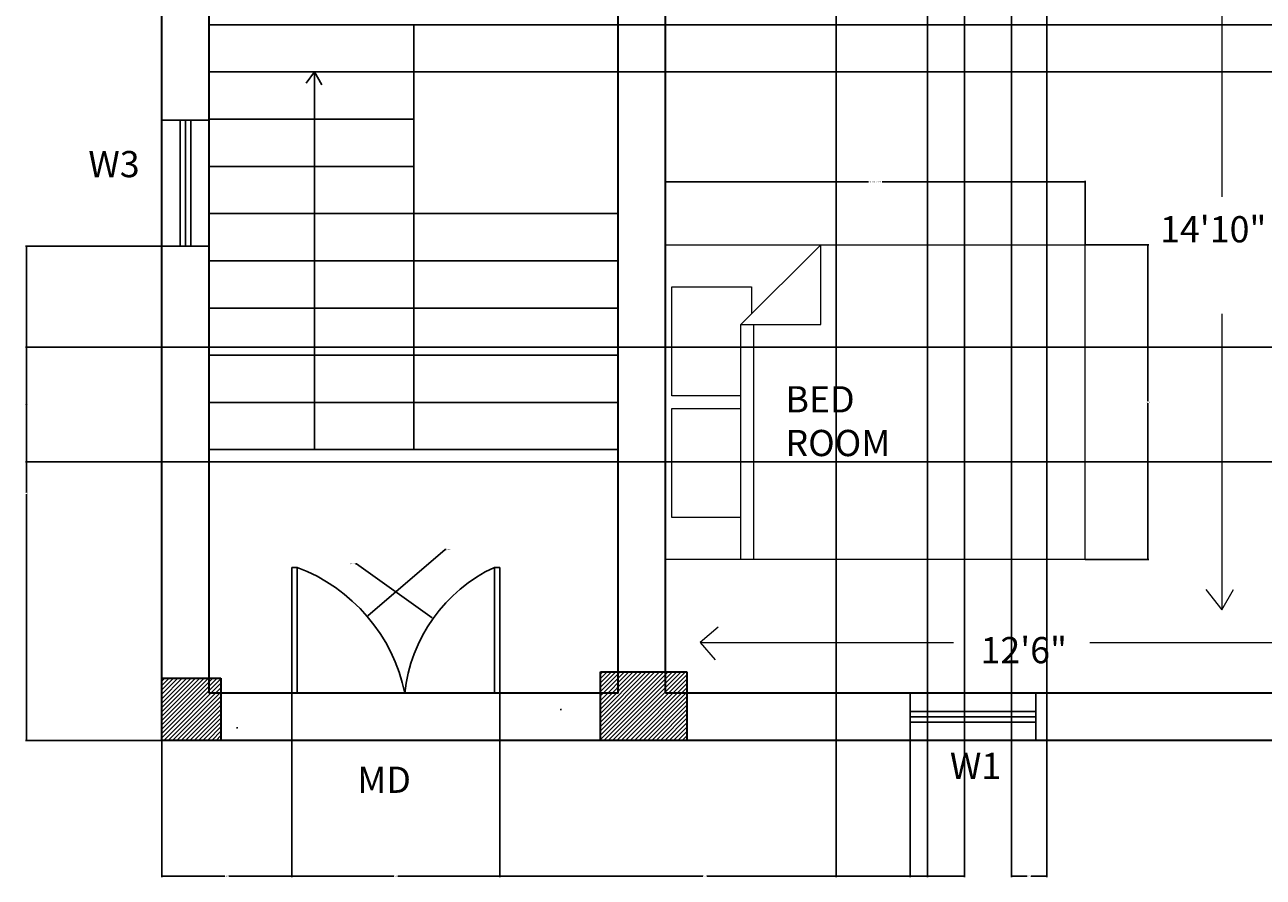
# Model space of a CAD drawing. Units: inches. Extents: x -4 to 429, y -457 to 84.
# Tile 1 of 4: x -4 to 232, y -457 to -295. Entities that reach past the tile are written whole.
import ezdxf

# ---------------------------------------------------------------- set-up
doc = ezdxf.new("R2010")
doc.units = ezdxf.units.IN
doc.header["$MEASUREMENT"] = 0
for name, color, linetype, lineweight in [('A-ANNO-DIMS', 2, 'Continuous', 18), ('A-ANNO-TEXT', 3, 'Continuous', 18), ('A-AREA-IDEN', 7, 'Continuous', 25), ('A-COLS', 7, 'Continuous', 35), ('A-COLS-PATT', 252, 'Continuous', 13), ('A-DOOR', 3, 'Continuous', 25), ('A-FLOR-STRS', 7, 'Continuous', 25), ('A-FURN', 8, 'Continuous', 18), ('A-GLAZ', 4, 'Continuous', 25), ('A-WALL', 7, 'Continuous', 35)]:
    doc.layers.add(name, color=color, linetype=linetype, lineweight=lineweight)
doc.styles.get("Standard").update_dxf_attribs({"font": 'arial.ttf'})
doc.dimstyles.get("Standard").update_dxf_attribs({"dimtxt": 0.18, "dimasz": 0.18, "dimexe": 0.18, "dimexo": 0.0625, "dimgap": 0.09, "dimtad": 0, "dimtih": 1, "dimtoh": 1, "dimdec": 4, "dimzin": 0, "dimdsep": 46, "dimtxsty": 'Standard', "dimcen": 0.09, "dimadec": 0, "dimazin": 0, "dimtfac": 1, "dimtdec": 4, "dimtofl": 0, "dimtmove": 0, "dimatfit": 3, "dimfxl": 1, "dimtolj": 1, "dimtzin": 0, "dimarcsym": 0})
pattern_1 = [(45, (-1330.13025, -719.5531), (-0.41542523, 0.41542523), [])]

# ---------------------------------------------------------------- blocks, each defined once
blk = doc.blocks.new('Bed - Queen')
for p, q in [((0, -80.00003), (0, 0)), ((0, 0), (59.99999, 0)), ((59.99999, 0), (59.99999, -80.00003)), ((7.99999, -1.2), (28.79998, -1.2)), ((7.99999, -14.4), (7.99999, -1.2)), ((28.79998, -1.2), (28.79998, -14.4)), ((31.19999, -1.2), (51.99999, -1.2)), ((31.19999, -14.4), (31.19999, -1.2)), ((51.99999, -1.2), (51.99999, -16.4)), ((0, -14.4), (44.8, -14.4)), ((59.99999, -29.6), (44.8, -14.4)), ((44.8, -14.4), (44.8, -29.6)), ((51.99999, -16.4), (46.79936, -16.4)), ((44.8, -16.8), (0, -16.8)), ((44.8, -29.6), (59.99999, -29.6)), ((59.99999, -80.00003), (0, -80.00003))]:
    blk.add_line(p, q)
blk = doc.blocks.new('WIN-24IN-9IN-WALL')
for p, q in [((0, 5.5), (24, 5.5)), ((0, 4.5), (24, 4.5)), ((0, 3.5), (24, 3.5))]:
    blk.add_line(p, q)
blk.add_lwpolyline([(0, 9), (24, 9), (24, 0), (0, 0)], close=True)
blk = doc.blocks.new('DOOR-LEAF-24IN')
for p, q in [((0, 0), (0, 24)), ((0, 24), (1, 24)), ((1, 24), (1, 0))]:
    blk.add_line(p, q)
blk = doc.blocks.new('*D16')
at = {"layer": 'A-ANNO-DIMS', "color": 0, "lineweight": -2, "transparency": 16777216}
for p, q in [((118.06, -336.78), (118.06, -324.66)), ((118.24, -324.84), (156.75, -324.84)), ((197.88, -324.84), (159.36, -324.84)), ((198.06, -336.78), (198.06, -324.66))]:
    blk.add_line(p, q, dxfattribs=at)
at = {"layer": 'A-ANNO-DIMS', "color": 0, "transparency": 16777216}
for points in [[(118.24, -324.81), (118.24, -324.87), (118.06, -324.84)], [(197.88, -324.81), (197.88, -324.87), (198.06, -324.84)]]:
    blk.add_solid(points, dxfattribs=at)
at = {"layer": 'Defpoints', "color": 0, "transparency": 16777216}
for p in [(118.06, -324.84), (118.06, -336.84), (198.06, -336.84)]:
    blk.add_point(p, dxfattribs=at)
at = {"layer": 'A-ANNO-DIMS', "color": 0, "transparency": 16777216, "insert": (158.06, -324.84), "char_height": 0.18, "attachment_point": 5}
blk.add_mtext('\\A1;QUEEN BED 80 TYP.', dxfattribs=at)
blk = doc.blocks.new('*D17')
at = {"layer": 'A-ANNO-DIMS', "color": 0, "lineweight": -2, "transparency": 16777216}
for p, q in [((198.12, -336.84), (210.24, -336.84)), ((210.06, -337.02), (210.06, -366.66)), ((210.06, -396.66), (210.06, -367.02)), ((198.12, -396.84), (210.24, -396.84))]:
    blk.add_line(p, q, dxfattribs=at)
at = {"layer": 'A-ANNO-DIMS', "color": 0, "transparency": 16777216}
for points in [[(210.03, -337.02), (210.09, -337.02), (210.06, -336.84)], [(210.03, -396.66), (210.09, -396.66), (210.06, -396.84)]]:
    blk.add_solid(points, dxfattribs=at)
at = {"layer": 'Defpoints', "color": 0, "transparency": 16777216}
for p in [(198.06, -336.84), (210.06, -336.84), (198.06, -396.84)]:
    blk.add_point(p, dxfattribs=at)
at = {"layer": 'A-ANNO-DIMS', "color": 0, "transparency": 16777216, "insert": (210.06, -366.84), "char_height": 0.18, "attachment_point": 5}
blk.add_mtext('\\A1;60 TYP.', dxfattribs=at)
blk = doc.blocks.new('*D33')
at = {"layer": 'A-ANNO-DIMS', "color": 0, "lineweight": -2, "transparency": 16777216}
for p, q in [((70.12, -294.9), (429.31, -294.9)), ((429.13, -295.08), (429.13, -299.22)), ((429.13, -303.72), (429.13, -299.59)), ((70.12, -303.9), (429.31, -303.9))]:
    blk.add_line(p, q, dxfattribs=at)
at = {"layer": 'A-ANNO-DIMS', "color": 0, "transparency": 16777216}
for points in [[(429.1, -295.08), (429.16, -295.08), (429.13, -294.9)], [(429.1, -303.72), (429.16, -303.72), (429.13, -303.9)]]:
    blk.add_solid(points, dxfattribs=at)
at = {"layer": 'Defpoints', "color": 0, "transparency": 16777216}
for p in [(70.06, -294.9), (70.06, -303.9), (429.13, -303.9)]:
    blk.add_point(p, dxfattribs=at)
at = {"layer": 'A-ANNO-DIMS', "color": 0, "transparency": 16777216, "insert": (429.13, -299.4), "char_height": 0.18, "attachment_point": 5}
blk.add_mtext('\\A1;9', dxfattribs=at)
blk = doc.blocks.new('*D35')
at = {"layer": 'A-ANNO-DIMS', "color": 0, "lineweight": -2, "transparency": 16777216}
for p, q in [((150.6, -85.07), (150.6, -457.42)), ((175.06, -85.07), (175.06, -457.42)), ((150.78, -457.24), (162.36, -457.24)), ((174.88, -457.24), (163.29, -457.24))]:
    blk.add_line(p, q, dxfattribs=at)
at = {"layer": 'A-ANNO-DIMS', "color": 0, "transparency": 16777216}
for points in [[(150.78, -457.21), (150.78, -457.27), (150.6, -457.24)], [(174.88, -457.21), (174.88, -457.27), (175.06, -457.24)]]:
    blk.add_solid(points, dxfattribs=at)
at = {"layer": 'Defpoints', "color": 0, "transparency": 16777216}
for p in [(150.6, -85.01), (175.06, -85.01), (175.06, -457.24)]:
    blk.add_point(p, dxfattribs=at)
at = {"layer": 'A-ANNO-DIMS', "color": 0, "transparency": 16777216, "insert": (162.83, -457.24), "char_height": 0.18, "attachment_point": 5}
blk.add_mtext('\\A1;24.457', dxfattribs=at)
blk = doc.blocks.new('*D42')
at = {"layer": 'A-ANNO-DIMS', "color": 0, "lineweight": -2, "transparency": 16777216}
for p, q in [((324.99, -356.34), (-3.97, -356.34)), ((-3.79, -356.52), (-3.79, -367.09)), ((-3.79, -378.03), (-3.79, -367.46)), ((324.99, -378.21), (-3.97, -378.21))]:
    blk.add_line(p, q, dxfattribs=at)
at = {"layer": 'A-ANNO-DIMS', "color": 0, "transparency": 16777216}
for points in [[(-3.82, -356.52), (-3.76, -356.52), (-3.79, -356.34)], [(-3.82, -378.03), (-3.76, -378.03), (-3.79, -378.21)]]:
    blk.add_solid(points, dxfattribs=at)
at = {"layer": 'Defpoints', "color": 0, "transparency": 16777216}
for p in [(325.06, -356.34), (-3.79, -378.21), (325.06, -378.21)]:
    blk.add_point(p, dxfattribs=at)
at = {"layer": 'A-ANNO-DIMS', "color": 0, "transparency": 16777216, "insert": (-3.79, -367.28), "char_height": 0.18, "attachment_point": 5}
blk.add_mtext('\\A1;21.87', dxfattribs=at)
blk = doc.blocks.new('*D44')
at = {"layer": 'A-ANNO-DIMS', "color": 0, "lineweight": -2, "transparency": 16777216}
for p, q in [((21.99, -337.11), (-3.97, -337.11)), ((-3.79, -337.29), (-3.79, -384.04)), ((-3.79, -431.16), (-3.79, -384.41)), ((21.99, -431.34), (-3.97, -431.34))]:
    blk.add_line(p, q, dxfattribs=at)
at = {"layer": 'A-ANNO-DIMS', "color": 0, "transparency": 16777216}
for points in [[(-3.82, -337.29), (-3.76, -337.29), (-3.79, -337.11)], [(-3.82, -431.16), (-3.76, -431.16), (-3.79, -431.34)]]:
    blk.add_solid(points, dxfattribs=at)
at = {"layer": 'Defpoints', "color": 0, "transparency": 16777216}
for p in [(22.06, -337.11), (-3.79, -431.34), (22.06, -431.34)]:
    blk.add_point(p, dxfattribs=at)
at = {"layer": 'A-ANNO-DIMS', "color": 0, "transparency": 16777216, "insert": (-3.79, -384.22), "char_height": 0.18, "attachment_point": 5}
blk.add_mtext('\\A1;94.23', dxfattribs=at)
blk = doc.blocks.new('*D45')
at = {"layer": 'A-ANNO-DIMS', "color": 0, "lineweight": -2, "transparency": 16777216}
for p, q in [((22.06, -419.56), (22.06, -457.42)), ((46.84, -422.4), (46.84, -457.42)), ((22.24, -457.24), (34.05, -457.24)), ((46.66, -457.24), (34.84, -457.24))]:
    blk.add_line(p, q, dxfattribs=at)
at = {"layer": 'A-ANNO-DIMS', "color": 0, "transparency": 16777216}
for points in [[(22.24, -457.21), (22.24, -457.27), (22.06, -457.24)], [(46.66, -457.21), (46.66, -457.27), (46.84, -457.24)]]:
    blk.add_solid(points, dxfattribs=at)
at = {"layer": 'Defpoints', "color": 0, "transparency": 16777216}
for p in [(22.06, -419.49), (46.84, -422.34), (46.84, -457.24)]:
    blk.add_point(p, dxfattribs=at)
at = {"layer": 'A-ANNO-DIMS', "color": 0, "transparency": 16777216, "insert": (34.45, -457.24), "char_height": 0.18, "attachment_point": 5}
blk.add_mtext('\\A1;24.78', dxfattribs=at)
blk = doc.blocks.new('*D46')
at = {"layer": 'A-ANNO-DIMS', "color": 0, "lineweight": -2, "transparency": 16777216}
for p, q in [((46.84, -422.4), (46.84, -457.42)), ((86.46, -422.4), (86.46, -457.42)), ((47.02, -457.24), (66.26, -457.24)), ((86.28, -457.24), (67.04, -457.24))]:
    blk.add_line(p, q, dxfattribs=at)
at = {"layer": 'A-ANNO-DIMS', "color": 0, "transparency": 16777216}
for points in [[(47.02, -457.21), (47.02, -457.27), (46.84, -457.24)], [(86.28, -457.21), (86.28, -457.27), (86.46, -457.24)]]:
    blk.add_solid(points, dxfattribs=at)
at = {"layer": 'Defpoints', "color": 0, "transparency": 16777216}
for p in [(46.84, -422.34), (86.46, -422.34), (86.46, -457.24)]:
    blk.add_point(p, dxfattribs=at)
at = {"layer": 'A-ANNO-DIMS', "color": 0, "transparency": 16777216, "insert": (66.65, -457.24), "char_height": 0.18, "attachment_point": 5}
blk.add_mtext('\\A1;39.63', dxfattribs=at)
blk = doc.blocks.new('*D47')
at = {"layer": 'A-ANNO-DIMS', "color": 0, "lineweight": -2, "transparency": 16777216}
for p, q in [((86.46, -422.4), (86.46, -457.42)), ((164.71, -431.4), (164.71, -457.42)), ((86.64, -457.24), (125.19, -457.24)), ((164.53, -457.24), (125.98, -457.24))]:
    blk.add_line(p, q, dxfattribs=at)
at = {"layer": 'A-ANNO-DIMS', "color": 0, "transparency": 16777216}
for points in [[(86.64, -457.21), (86.64, -457.27), (86.46, -457.24)], [(164.53, -457.21), (164.53, -457.27), (164.71, -457.24)]]:
    blk.add_solid(points, dxfattribs=at)
at = {"layer": 'Defpoints', "color": 0, "transparency": 16777216}
for p in [(86.46, -422.34), (164.71, -431.34), (164.71, -457.24)]:
    blk.add_point(p, dxfattribs=at)
at = {"layer": 'A-ANNO-DIMS', "color": 0, "transparency": 16777216, "insert": (125.59, -457.24), "char_height": 0.18, "attachment_point": 5}
blk.add_mtext('\\A1;78.25', dxfattribs=at)
blk = doc.blocks.new('*D51')
at = {"layer": 'A-ANNO-DIMS', "color": 0, "lineweight": -2, "transparency": 16777216}
for p, q in [((175.06, -118.1), (175.06, -457.42)), ((168.05, -122.4), (168.05, -457.42)), ((168.23, -457.24), (171.16, -457.24)), ((174.88, -457.24), (171.95, -457.24))]:
    blk.add_line(p, q, dxfattribs=at)
at = {"layer": 'A-ANNO-DIMS', "color": 0, "transparency": 16777216}
for points in [[(168.23, -457.21), (168.23, -457.27), (168.05, -457.24)], [(174.88, -457.21), (174.88, -457.27), (175.06, -457.24)]]:
    blk.add_solid(points, dxfattribs=at)
at = {"layer": 'Defpoints', "color": 0, "transparency": 16777216}
for p in [(175.06, -118.04), (168.05, -122.34), (175.06, -457.24)]:
    blk.add_point(p, dxfattribs=at)
at = {"layer": 'A-ANNO-DIMS', "color": 0, "transparency": 16777216, "insert": (171.56, -457.24), "char_height": 0.18, "attachment_point": 5}
blk.add_mtext('\\A1;7.002', dxfattribs=at)
blk = doc.blocks.new('*D52')
at = {"layer": 'A-ANNO-DIMS', "color": 0, "lineweight": -2, "transparency": 16777216}
for p, q in [((184.06, -118.1), (184.06, -457.42)), ((190.77, -122.4), (190.77, -457.42)), ((184.24, -457.24), (187.02, -457.24)), ((190.59, -457.24), (187.81, -457.24))]:
    blk.add_line(p, q, dxfattribs=at)
at = {"layer": 'A-ANNO-DIMS', "color": 0, "transparency": 16777216}
for points in [[(184.24, -457.21), (184.24, -457.27), (184.06, -457.24)], [(190.59, -457.21), (190.59, -457.27), (190.77, -457.24)]]:
    blk.add_solid(points, dxfattribs=at)
at = {"layer": 'Defpoints', "color": 0, "transparency": 16777216}
for p in [(184.06, -118.04), (190.77, -122.34), (190.77, -457.24)]:
    blk.add_point(p, dxfattribs=at)
at = {"layer": 'A-ANNO-DIMS', "color": 0, "transparency": 16777216, "insert": (187.41, -457.24), "char_height": 0.18, "attachment_point": 5}
blk.add_mtext('\\A1;6.714', dxfattribs=at)
blk = doc.blocks.new('*D53')
at = {"layer": 'A-ANNO-DIMS', "color": 0, "lineweight": -2, "transparency": 16777216}
for p, q in [((76.08, -394.96), (61.33, -407.57)), ((76.26, -394.96), (76.08, -394.96)), ((36.29, -428.92), (36.47, -428.92)), ((36.38, -429.01), (36.38, -428.83))]:
    blk.add_line(p, q, dxfattribs=at)
at = {"layer": 'A-ANNO-DIMS', "color": 0, "transparency": 16777216}
blk.add_solid([(61.31, -407.55), (61.35, -407.6), (61.2, -407.69)], dxfattribs=at)
at = {"layer": 'Defpoints', "color": 0, "transparency": 16777216}
for p in [(61.2, -407.69), (36.38, -428.92)]:
    blk.add_point(p, dxfattribs=at)
at = {"layer": 'A-ANNO-DIMS', "color": 0, "transparency": 16777216, "insert": (76.81, -394.96), "char_height": 0.18, "attachment_point": 5}
blk.add_mtext('\\A1;R32.654', dxfattribs=at)
blk = doc.blocks.new('*D54')
at = {"layer": 'A-ANNO-DIMS', "color": 0, "lineweight": -2, "transparency": 16777216}
for p, q in [((58.96, -397.68), (59.14, -397.68)), ((59.14, -397.68), (73.61, -407.98)), ((98.03, -425.45), (98.21, -425.45)), ((98.12, -425.54), (98.12, -425.36))]:
    blk.add_line(p, q, dxfattribs=at)
at = {"layer": 'A-ANNO-DIMS', "color": 0, "transparency": 16777216}
blk.add_solid([(73.63, -407.96), (73.59, -408.01), (73.76, -408.09)], dxfattribs=at)
at = {"layer": 'Defpoints', "color": 0, "transparency": 16777216}
for p in [(73.76, -408.09), (98.12, -425.45)]:
    blk.add_point(p, dxfattribs=at)
at = {"layer": 'A-ANNO-DIMS', "color": 0, "transparency": 16777216, "insert": (58.41, -397.68), "char_height": 0.18, "attachment_point": 5}
blk.add_mtext('\\A1;R29.917', dxfattribs=at)

msp = doc.modelspace()

# ---------------------------------------------------------------- hatches: boundary and pattern name
at = {"layer": 'A-COLS-PATT'}
h = msp.add_hatch(dxfattribs=at)
h.set_pattern_fill('ANSI31', color=256, scale=4.7)
h.set_pattern_definition(pattern_1)
h.paths.add_polyline_path([(33.2927, -422.3399), (31.0572, -422.3399), (31.0572, -419.4944), (22.0572, -419.4944), (22.0572, -431.3399), (33.2927, -431.3399)])
h.paths.add_polyline_path([(33.2927, -419.4944), (31.0572, -419.4944), (31.0572, -422.3399), (33.2927, -422.3399)], flags=17)
h = msp.add_hatch(dxfattribs=at)
h.set_pattern_fill('ANSI31', color=256, scale=4.7)
h.set_pattern_definition(pattern_1)
h.paths.add_polyline_path([(109.0572, -418.2666), (105.6558, -418.2666), (105.6558, -422.3399), (109.0572, -422.3399)], flags=17)
h.paths.add_polyline_path([(122.1688, -422.3399), (118.0572, -422.3399), (118.0572, -418.2666), (109.0572, -418.2666), (109.0572, -422.3399), (105.6558, -422.3399), (105.6558, -431.3399), (122.1688, -431.3399)])
h.paths.add_polyline_path([(122.1688, -418.2666), (118.0572, -418.2666), (118.0572, -422.3399), (122.1688, -422.3399)], flags=17)

# ---------------------------------------------------------------- linework, layer by layer
at = {"layer": 'A-ANNO-DIMS'}
for p, q in [((224.1656, -269.5865), (224.1656, -327.7164)), ((224.1656, -349.979), (224.1656, -406.4598)), ((221.1061, -402.5517), (224.1656, -406.4598)), ((224.1656, -406.4598), (226.3996, -402.5905)), ((128.1382, -409.7303), (124.6924, -412.6439)), ((124.6924, -412.6439), (172.9844, -412.6439)), ((124.6924, -412.6439), (127.5215, -415.9899)), ((198.9877, -412.6439), (247.6925, -412.6439))]:
    msp.add_line(p, q, dxfattribs=at)
at = {"layer": 'A-COLS'}
for p, q in [((22.0572, -419.4944), (33.2927, -419.4944)), ((33.2927, -419.4944), (33.2927, -431.3399)), ((105.6558, -431.3399), (105.6558, -418.2666)), ((105.6558, -418.2666), (122.1688, -418.2666)), ((122.1688, -418.2666), (122.1688, -431.3399))]:
    msp.add_line(p, q, dxfattribs=at)
at = {"layer": 'A-DOOR'}
for centre, radius, start, end in [((36.3849, -428.9199), 32.6537, 11.625121, 69.470881), ((98.1237, -425.4453), 29.9165, 115.03719, 174.041898)]:
    msp.add_arc(centre, radius, start, end, dxfattribs=at)
at = {"layer": 'A-FLOR-STRS'}
for p, q in [((70.0572, -294.9035), (31.0572, -294.9035)), ((70.0572, -298.1185), (70.0572, -294.9035)), ((70.0572, -298.1185), (70.0572, -375.9035)), ((70.0572, -303.9035), (31.0572, -303.9035)), ((49.5596, -306.0463), (51.1539, -303.9035)), ((51.1539, -375.9035), (51.1539, -303.9035)), ((51.1539, -303.9035), (52.5562, -306.3324)), ((70.0572, -312.9035), (31.0572, -312.9035)), ((70.0572, -321.9035), (31.0572, -321.9035)), ((109.0572, -330.9035), (31.0572, -330.9035)), ((109.0572, -339.9035), (31.0572, -339.9035)), ((109.0572, -348.9035), (31.0572, -348.9035)), ((109.0572, -357.9035), (31.0572, -357.9035)), ((109.0572, -366.9035), (31.0572, -366.9035)), ((109.0572, -375.9035), (31.0572, -375.9035))]:
    msp.add_line(p, q, dxfattribs=at)
at = {"layer": 'A-WALL'}
for p, q in [((109.0572, -422.3399), (109.0572, -251.3399)), ((118.0572, -422.3399), (118.0572, -251.3399)), ((31.0572, -422.3399), (31.0572, -260.3399)), ((109.0572, -422.3399), (31.0572, -422.3399)), ((252.0572, -422.3399), (118.0572, -422.3399))]:
    msp.add_line(p, q, dxfattribs=at)
msp.add_lwpolyline([(22.0572, 18.6601), (334.0572, 18.6601), (334.0572, -431.3399), (22.0572, -431.3399)], close=True, dxfattribs=at)

# ---------------------------------------------------------------- block references
at = {"layer": 'A-DOOR'}
for p in [(46.8358, -422.34), (85.4626, -422.34)]:
    msp.add_blockref('DOOR-LEAF-24IN', p, dxfattribs=at)
at = {"layer": 'A-FURN', "rotation": 90}
msp.add_blockref('Bed - Queen', (118.0572, -396.8399), dxfattribs=at)
at = {"layer": 'A-GLAZ', "extrusion": (0, 0, -1), "zscale": -1, "rotation": 270}
msp.add_blockref('WIN-24IN-9IN-WALL', (-31.0573, -313.1087), dxfattribs=at)
at = {"layer": 'A-GLAZ'}
msp.add_blockref('WIN-24IN-9IN-WALL', (164.7081, -431.34), dxfattribs=at)

# ---------------------------------------------------------------- texts
at = {"layer": 'A-ANNO-DIMS', "char_height": 5, "attachment_point": 1}
for s, width, insert in [('14\'10"', 24.738309, (212.3735, -331.3867)), ('12\'6"', 20.907462, (178.1371, -411.6207))]:
    msp.add_mtext_dynamic_manual_height_columns(s, width=width, gutter_width=25, heights=[0], dxfattribs=dict(at, insert=insert))
at = {"layer": 'A-ANNO-TEXT', "char_height": 5, "attachment_point": 1}
for s, width, insert in [('W3', 11.271693, (8.0256, -318.9662)), ('W1', 58.615968, (172.3037, -433.7015)), ('MD', 36.262423, (59.3057, -436.3399))]:
    msp.add_mtext_dynamic_manual_height_columns(s, width=width, gutter_width=25, heights=[0], dxfattribs=dict(at, insert=insert))
at = {"layer": 'A-AREA-IDEN', "insert": (140.9436, -363.8019), "char_height": 5, "attachment_point": 1}
msp.add_mtext_dynamic_manual_height_columns('BED\\PROOM', width=37.20908, gutter_width=25, heights=[0], dxfattribs=at)

# ---------------------------------------------------------------- dimensions: what is measured, and where the dimension line sits
at = {"layer": 'A-ANNO-DIMS'}
for base, p1, p2, override, picture, middle in [((175.0572, -457.2361), (150.6, -85.0072), (175.0572, -85.0072), {"dimdec": 3, "dimlfac": 1, "dimrnd": 0, "dimzin": 0, "dimdsep": 46, "dimlunit": 2}, '*D35', (162.8286, -457.2361)), ((175.0572, -457.2361), (168.0549, -122.3399), (175.0572, -118.0379), {"dimdec": 3, "dimlfac": 1, "dimrnd": 0, "dimzin": 0, "dimdsep": 46, "dimlunit": 2}, '*D51', (171.5561, -457.2361)), ((190.7712, -457.2361), (184.0572, -118.0379), (190.7712, -122.3399), {"dimdec": 3, "dimlfac": 1, "dimrnd": 0, "dimzin": 0, "dimdsep": 46, "dimlunit": 2}, '*D52', (187.4142, -457.2361)), ((46.836, -457.2361), (22.0572, -419.4944), (46.836, -422.3399), {"dimdec": 2, "dimlfac": 1, "dimrnd": 0, "dimzin": 0, "dimdsep": 46, "dimlunit": 2}, '*D45', (34.4466, -457.2361)), ((86.4628, -457.2361), (46.836, -422.3399), (86.4628, -422.3399), {"dimdec": 2, "dimlfac": 1, "dimrnd": 0, "dimzin": 0, "dimdsep": 46, "dimlunit": 2}, '*D46', (66.6494, -457.2361)), ((164.708, -457.2361), (86.4628, -422.3399), (164.708, -431.3399), {"dimdec": 2, "dimlfac": 1, "dimrnd": 0, "dimzin": 0, "dimdsep": 46, "dimlunit": 2}, '*D47', (125.5854, -457.2361))]:
    dim = msp.add_linear_dim(base=base, p1=p1, p2=p2, dimstyle='Standard', override=override, dxfattribs=at)
    dim.commit()
    dim.dimension.update_dxf_attribs({"geometry": picture, "text_midpoint": middle})
for base, p1, p2, override, picture, middle in [((429.1331, -303.9035), (70.0572, -294.9035), (70.0572, -303.9035), {"dimdec": 0, "dimlfac": 1, "dimrnd": 0, "dimzin": 0, "dimdsep": 46, "dimlunit": 2}, '*D33', (429.1331, -299.4035)), ((-3.7928, -431.3399), (22.0572, -337.1085), (22.0572, -431.3399), {"dimdec": 2, "dimlfac": 1, "dimrnd": 0, "dimzin": 0, "dimdsep": 46, "dimlunit": 2}, '*D44', (-3.7928, -384.2242)), ((-3.7928, -378.2115), (325.0572, -356.3399), (325.0572, -378.2115), {"dimdec": 2, "dimlfac": 1, "dimrnd": 0, "dimzin": 0, "dimdsep": 46, "dimlunit": 2}, '*D42', (-3.7928, -367.2757))]:
    dim = msp.add_linear_dim(base=base, p1=p1, p2=p2, angle=90, dimstyle='Standard', override=override, dxfattribs=at)
    dim.commit()
    dim.dimension.update_dxf_attribs({"geometry": picture, "text_midpoint": middle})
for base, p1, p2, angle, text, picture, middle in [((118.0572, -324.8399), (198.0573, -336.8399), (118.0572, -336.8399), 180, 'QUEEN BED <> TYP.', '*D16', (158.0573, -324.8399)), ((210.0573, -336.8399), (198.0573, -396.8399), (198.0573, -336.8399), 90, '<> TYP.', '*D17', (210.0573, -366.8399))]:
    dim = msp.add_linear_dim(base=base, p1=p1, p2=p2, angle=angle, text=text, dimstyle='Standard', override={"dimdec": 0, "dimlfac": 1, "dimrnd": 0, "dimzin": 0, "dimdsep": 46, "dimlunit": 2}, dxfattribs=at)
    dim.commit()
    dim.dimension.update_dxf_attribs({"geometry": picture, "text_midpoint": middle})
for center, mpoint, picture, middle in [((36.3849, -428.9199), (61.197, -407.692), '*D53', (76.8136, -394.9553)), ((98.1237, -425.4453), (73.7563, -408.0892), '*D54', (58.4062, -397.6756))]:
    dim = msp.add_radius_dim(center=center, mpoint=mpoint, dimstyle='Standard', override={"dimdec": 3, "dimlfac": 1, "dimrnd": 0, "dimzin": 0, "dimdsep": 46, "dimlunit": 2}, dxfattribs=at)
    dim.commit()
    dim.dimension.update_dxf_attribs({"geometry": picture, "text_midpoint": middle, "dimtype": 164})

doc.saveas('drawing.dxf')
